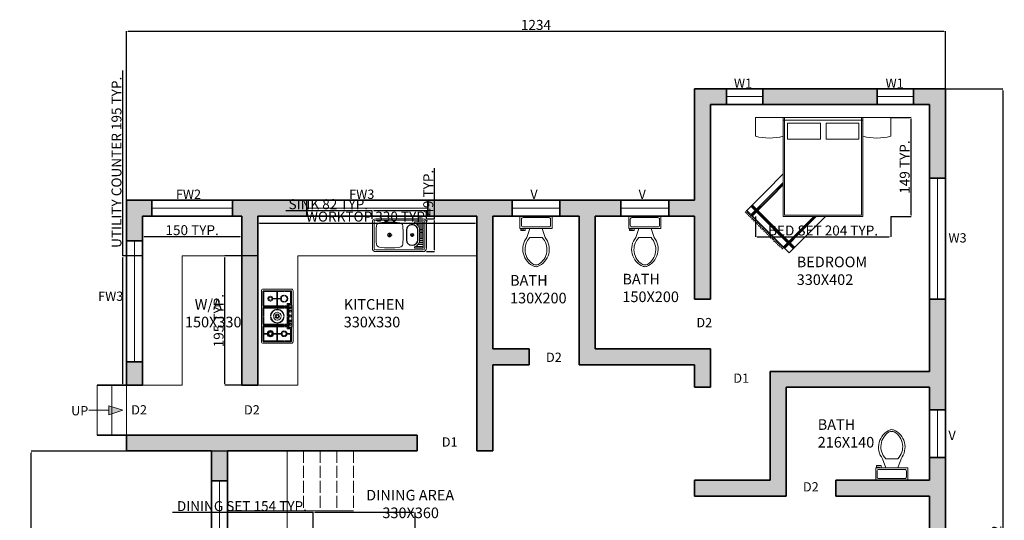
# Model space of a CAD drawing. Units: centimetres. Extents: x 2449 to 7478, y 778 to 2486.
# Tile 6 of 9: x 4189 to 5672, y 1732 to 2486. Entities that reach past the tile are written whole.
import ezdxf

# ---------------------------------------------------------------- set-up
doc = ezdxf.new("R2010")
doc.units = ezdxf.units.CM
doc.linetypes.add('ACAD_ISO02W100', pattern=[15, 12, -3])
for name, color, linetype, lineweight in [('A-ANNO-DIMS', 2, 'Continuous', 18), ('A-ANNO-SYMB', 8, 'Continuous', 18), ('A-ANNO-TEXT', 7, 'Continuous', 18), ('A-AREA-IDEN', 7, 'Continuous', 18), ('A-EQPM', 8, 'Continuous', 18), ('A-FLOR-CASE', 8, 'Continuous', 18), ('A-FLOR-FIXT', 8, 'Continuous', 18), ('A-FLOR-STRS', 7, 'Continuous', 18), ('A-FLOR-STRS-OVHD', 7, 'ACAD_ISO02W100', 13), ('A-WALL', 7, 'Continuous', 35), ('A-WALL-PATT', 7, 'Continuous', 13), ('B-FURNITURE', 22, 'Continuous', 18), ('Win', 1, 'Continuous', 18)]:
    doc.layers.add(name, color=color, linetype=linetype, lineweight=lineweight)
doc.styles.get("Standard").update_dxf_attribs({"font": 'arial.ttf'})
doc.dimstyles.new('ISO-25', dxfattribs={"dimtxt": 15, "dimasz": 2.5, "dimexe": 0, "dimexo": 0, "dimgap": 0, "dimtad": 1, "dimtxsty": 'Standard', "dimcen": 2.5, "dimadec": 0, "dimazin": 0, "dimtfac": 1, "dimtmove": 0, "dimatfit": 3, "dimfxl": 1, "dimarcsym": 0})

# ---------------------------------------------------------------- blocks, each defined once
blk = doc.blocks.new('sink 1')
for points in [[(-7.34, 1.48), (-7.34, 22.73)], [(-6.56, 1.48), (-6.56, 22.73)], [(5.86, 24.22), (-5.86, 24.22)], [(6.01, 23.43), (-5.86, 23.43)], [(6.72, 1.48), (6.72, 22.73)], [(7.34, 1.48), (7.34, 22.73)], [(1.09, 16.48), (-0.94, 16.48)], [(0, 15.39), (0, 17.42)], [(-2.09, 8.99), (2.28, 8.99)], [(-2.09, 8.84), (2.28, 8.84)], [(-5.78, 5.39), (-5.78, 5.39)], [(-5.31, 5.39), (-5.31, 5.39)], [(-5.16, 4.92), (-5.16, 4.92)], [(-5, 1.48), (-5, 4.69)], [(-4.84, 4.45), (-4.84, 4.45)], [(0.78, 6.33), (-0.78, 6.33)], [(0, 5.55), (0, 7.26)], [(5, 4.45), (5, 4.45)], [(5.16, 4.92), (5.16, 4.92)], [(5.94, 5.39), (5.94, 5.39)], [(6.01, 0.78), (-5.86, 0.78)], [(5.86, 0), (-5.86, 0)], [(-5.78, 1.48), (-5.78, 1.48)], [(-5.16, 1.48), (-5.16, 1.48)], [(-5, 1.48), (-4.22, 1.48), (-4.22, 3.83)], [(-4.84, 1.48), (-4.84, 1.48)], [(-4.22, 3.83), (-4.22, 3.83)], [(-4.22, 1.48), (-4.22, 1.48)], [(-4.06, 1.48), (-4.06, 3.69)], [(-4.06, 1.48), (-3.28, 1.48), (-3.28, 3.27)], [(-3.91, 3.52), (-3.91, 3.52)], [(-3.91, 1.48), (-3.91, 1.48)], [(-3.28, 3.2), (-3.28, 3.2)], [(-3.28, 1.48), (-3.28, 1.48)], [(-3.12, 3.2), (-3.12, 3.2)], [(-3.12, 1.48), (-3.12, 1.48)], [(-2.34, 3.05), (-2.34, 3.05)], [(-2.34, 1.48), (-2.34, 1.48)], [(-2.19, 3.05), (-2.19, 3.05)], [(-2.19, 1.48), (-2.19, 1.48)], [(-2.09, 3.99), (2.28, 3.99)], [(-2.09, 3.84), (2.28, 3.84)], [(-1.41, 3.05), (-1.41, 3.05)], [(-1.41, 1.48), (-1.41, 1.48)], [(-1.25, 3.05), (-1.25, 3.05)], [(-0.47, 1.48), (-1.25, 1.48), (-1.25, 3.05), (-0.47, 3.05)], [(-1.25, 1.48), (-1.25, 1.48)], [(-0.62, 3.05), (-0.62, 3.05)], [(-0.62, 1.48), (-0.62, 1.48)], [(-0.47, 1.48), (-0.47, 3.05)], [(-0.31, 3.05), (-0.31, 3.05)], [(0.47, 1.48), (-0.31, 1.48), (-0.31, 3.05), (0.47, 3.05)], [(-0.31, 1.48), (-0.31, 1.48)], [(0.31, 3.05), (0.31, 3.05)], [(0.31, 1.48), (0.31, 1.48)], [(0.47, 1.48), (0.47, 3.05)], [(0.62, 3.05), (0.62, 3.05)], [(0.62, 1.48), (0.62, 1.48)], [(1.25, 3.05), (1.25, 3.05)], [(1.25, 1.48), (1.25, 1.48)], [(1.56, 3.05), (1.56, 3.05)], [(1.56, 1.48), (1.56, 1.48)], [(2.19, 3.05), (2.19, 3.05)], [(2.19, 1.48), (2.19, 1.48)], [(2.5, 3.05), (2.5, 3.05)], [(2.5, 1.48), (2.5, 1.48)], [(3.12, 3.2), (3.12, 3.2)], [(3.12, 1.48), (3.12, 1.48)], [(3.28, 1.48), (4.06, 1.48), (4.06, 3.57)], [(3.28, 1.48), (3.28, 3.2)], [(3.44, 3.2), (3.44, 3.2)], [(3.44, 1.48), (3.44, 1.48)], [(4.06, 3.52), (4.06, 3.52)], [(4.06, 1.48), (4.06, 1.48)], [(4.22, 1.48), (4.22, 3.67)], [(4.37, 3.83), (4.37, 3.83)], [(4.37, 1.48), (4.37, 1.48)], [(5, 1.48), (5, 1.48)], [(5.16, 1.48), (5.16, 1.48)], [(5.94, 1.48), (5.94, 1.48)]]:
    blk.add_lwpolyline(points)
for points in [[(-5.16, 4.92), (-5.16, 1.48), (-5.78, 1.48), (-5.78, 5.39), (-5.31, 5.39, -0.068511), (-5.16, 4.92)], [(4.22, 1.48), (5, 1.48), (5, 4.45, -0.083542), (4.22, 3.67, -0.083542)], [(5.16, 4.92, 0.248301), (5.47, 5.39), (5.94, 5.39), (5.94, 1.48), (5.16, 1.48), (5.16, 4.92)], [(4.06, 3.57, -0.061679), (3.32, 3.22)]]:
    blk.add_lwpolyline(points, format="xyb")
for points in [[(-3.12, 3.22), (-3.12, 1.48), (-2.34, 1.48), (-2.34, 3.05, -0.06228)], [(2.5, 3.05), (2.5, 1.48), (3.12, 1.48), (3.12, 3.2, -0.050256)]]:
    blk.add_lwpolyline(points, format="xyb", close=True)
for points in [[(-2.19, 3.05), (-1.41, 3.05), (-1.41, 1.48), (-2.19, 1.48)], [(0.62, 3.05), (1.25, 3.05), (1.25, 1.48), (0.62, 1.48)], [(2.19, 1.48), (2.19, 3.05), (1.56, 3.05), (1.56, 1.48)]]:
    blk.add_lwpolyline(points, close=True)
for centre, radius in [((0.09, 16.57), 0.859), ((0.09, 16.57), 0.703), ((0.09, 6.41), 0.703), ((0.09, 6.41), 0.547)]:
    blk.add_circle(centre, radius)
for centre, radius, start, end in [((-5.86, 22.73), 1.48, 90, 180), ((-5.86, 22.73), 0.703, 90, 180), ((-3.87, 20.82), 1.53, 97.3256, 171.1849), ((0.09, -12.65), 35.23, 83.2159, 96.7841), ((4.06, 20.82), 1.53, 8.8151, 82.6744), ((5.86, 22.73), 1.48, 360, 90), ((6.01, 22.73), 0.703, 0, 90), ((30.19, 16.56), 35.85, 172.7947, 187.4213), ((-30, 16.56), 35.85, 352.5787, 7.2053), ((-3.89, 12.12), 1.48, 187.4212, 263.2159), ((-2.1, 6.41), 2.58, 90, 270), ((-2.1, 6.41), 2.42, 90, 270), ((0.09, 45.63), 35.23, 263.2159, 276.7841), ((2.28, 6.41), 2.58, 270, 90), ((2.28, 6.41), 2.42, 270, 90), ((4.08, 12.12), 1.48, 276.7841, 352.5788), ((-2.15, 6.48), 3.36, 212.1095, 232.0862), ((-5.86, 1.48), 1.48, 180, 270), ((-5.86, 1.48), 0.703, 180, 270), ((-2.1, 6.41), 3.36, 234.156, 249.3275), ((2.14, 6.36), 3.36, 289.8633, 290.5971), ((5.86, 1.48), 1.48, 270, 0), ((6.01, 1.48), 0.703, 270, 360)]:
    blk.add_arc(centre, radius, start, end)
blk = doc.blocks.new('STOVE')
for p, q in [((11.85, 19.7), (11.55, 19.7)), ((11.55, 16.92), (11.55, 19.7)), ((11.85, 16.92), (11.85, 19.7)), ((-11.85, 13.73), (-11.85, 7.62)), ((-11.85, 13.73), (-11.55, 13.73)), ((-11.55, 13.73), (-11.55, 7.62)), ((11.85, 16.92), (11.55, 16.92)), ((11.85, 13.23), (11.55, 13.23)), ((11.55, 13.23), (11.55, 7.57)), ((11.85, 13.23), (11.85, 7.57)), ((-11.85, 10.75), (-16.4, 10.75)), ((-11.85, 10.25), (-16.4, 10.25)), ((-11.85, 7.62), (-11.55, 7.62)), ((-7, 10.75), (-11.55, 10.75)), ((-7, 10.25), (-11.55, 10.25)), ((7, 10.75), (11.55, 10.75)), ((7, 10.25), (11.55, 10.25)), ((11.85, 7.57), (11.55, 7.57)), ((11.85, 10.75), (16.4, 10.75)), ((11.85, 10.25), (16.4, 10.25)), ((-7, 3.9), (-8.4, 3.9)), ((-7.8, 3.3), (-7.8, 1)), ((-6.4, 3.3), (-7.8, 3.3)), ((7.3, 2.8), (-7.3, 2.8)), ((-7.3, 2.8), (-7.3, 0.8)), ((7.3, 0.8), (-7.3, 0.8)), ((-5.4, 3.9), (-6, 3.9)), ((-5.4, 3.9), (-0.15, 3.9)), ((0.15, 3.9), (5.4, 3.9)), ((6.4, 3.3), (7.8, 3.3)), ((7, 3.9), (8.4, 3.9)), ((7.3, 2.8), (7.3, 0.8)), ((7.8, 3.3), (7.8, 1)), ((8.4, 3.9), (8.4, 1.6)), ((11.85, 4.28), (11.55, 4.28)), ((11.55, 4.28), (11.55, 1.3)), ((11.85, 1.3), (11.55, 1.3)), ((11.85, 4.28), (11.85, 1.3))]:
    blk.add_line(p, q)
for points in [[(-17, 21), (17, 21, -0.414214), (18, 20), (18, 1, -0.414214), (17, 0), (-17, 0, -0.414214), (-18, 1), (-18, 20, -0.414214)], [(6, 3.3), (-6, 3.3), (-6, 19.4, -0.414214), (-5.4, 20), (5.4, 20, -0.414214), (6, 19.4)]]:
    blk.add_lwpolyline(points, format="xyb", close=True)
for points in [[(-7.8, 1), (-16.4, 1, -0.414214), (-17, 1.6), (-17, 19.4, -0.414214), (-16.4, 20), (-7, 20, -0.414214), (-6.4, 19.4), (-6.4, 3.3)], [(6.4, 19.4, -0.414214), (7, 20), (16.4, 20, -0.414214), (17, 19.4), (17, 1.6, -0.414214), (16.4, 1), (7.8, 1)]]:
    blk.add_lwpolyline(points, format="xyb")
for points in [[(-16.4, 15.22), (-16.4, 19.4), (-11.85, 19.4)], [(-16.4, 6.08), (-16.4, 14.92)], [(-11.55, 19.4), (-7, 19.4), (-7, 15.22)], [(-7, 14.92), (-7, 6.08)], [(-5.4, 15.22), (-5.4, 19.4), (-0.15, 19.4)], [(-5.4, 10.65), (-5.4, 14.92)], [(0.15, 19.4), (5.4, 19.4), (5.4, 15.22)], [(5.4, 14.92), (5.4, 10.65)], [(6.4, 3.3), (6.4, 19.4)], [(7, 15.22), (7, 19.4), (11.55, 19.4)], [(7, 6.08), (7, 14.92)], [(11.85, 19.4), (16.4, 19.4), (16.4, 15.22)], [(16.4, 14.92), (16.4, 6.08)], [(-5.4, 6.08), (-5.4, 10.35)], [(5.4, 10.35), (5.4, 6.08)], [(-11.85, 1.6), (-16.4, 1.6), (-16.4, 5.77)], [(-8.4, 3.9), (-8.4, 1.6), (-11.55, 1.6)], [(-7, 5.77), (-7, 3.9)], [(-5.4, 3.9), (-5.4, 5.77)], [(5.4, 5.77), (5.4, 3.9)], [(7, 3.9), (7, 5.77)], [(11.55, 1.6), (8.4, 1.6)], [(16.4, 5.77), (16.4, 1.6), (11.85, 1.6)]]:
    blk.add_lwpolyline(points)
for centre, radius in [((-11.7, 15.07), 1.1), ((11.7, 15.07), 1.6), ((11.7, 15.07), 1.1), ((0, 10.5), 1.4), ((0, 10.5), 0.8), ((11.7, 5.93), 1.4), ((-5.49, 1.8), 0.6), ((-3.3, 1.8), 0.6), ((0, 1.8), 0.6), ((3.39, 1.8), 0.6), ((5.57, 1.8), 0.6)]:
    blk.add_circle(centre, radius)
for centre, radius, start, end in [((-11.7, 15.07), 1.6, 95.37938, 174.62062), ((-11.7, 15.07), 1.6, 185.37938, 264.62062), ((-11.7, 15.07), 1.6, 5.37938, 84.62062), ((-11.7, 15.07), 1.6, 275.37938, 354.62062), ((0, 10.5), 4.6, 91.86867, 178.13133), ((0, 10.5), 4.3, 91.9991, 178.0009), ((0, 10.5), 4.6, 1.86867, 88.13133), ((0, 10.5), 4.3, 1.9991, 88.0009), ((11.7, 15.07), 2.1, 94.09604, 175.90396), ((11.7, 15.07), 2.1, 184.09604, 265.90396), ((11.7, 15.07), 2.1, 4.09604, 85.90396), ((11.7, 15.07), 2.1, 274.09604, 355.90396), ((-11.7, 5.93), 2.4, 93.58332, 176.41668), ((-11.7, 5.93), 2, 94.30122, 175.69878), ((-11.7, 5.93), 2.4, 3.58332, 86.41668), ((-11.7, 5.93), 2, 4.30122, 85.69878), ((0, 10.5), 4.6, 181.86867, 268.13133), ((0, 10.5), 4.3, 181.9991, 268.0009), ((0, 10.5), 2.6, 93.30736, 176.69264), ((0, 10.5), 2.6, 183.30736, 266.69264), ((0, 10.5), 2.6, 3.30736, 86.69264), ((0, 10.5), 4.6, 271.86867, 358.13133), ((0, 10.5), 4.3, 271.9991, 358.0009), ((0, 10.5), 2.6, 273.30736, 356.69264), ((11.7, 5.93), 1.9, 94.52806, 175.47194), ((11.7, 5.93), 1.9, 4.52806, 85.47194), ((-11.7, 5.93), 2.4, 183.58332, 266.41668), ((-11.7, 5.93), 2, 184.30122, 265.69878), ((-11.7, 5.93), 2.4, 273.58332, 356.41668), ((-11.7, 5.93), 2, 274.30122, 355.69878), ((-5.49, 1.8), 0.846, 89.99794, 270), ((-3.3, 1.8), 0.846, 89.99794, 270), ((0, 1.8), 0.846, 89.99794, 270), ((3.39, 1.8), 0.846, 89.99794, 270), ((5.57, 1.8), 0.846, 89.99794, 270), ((11.7, 5.93), 1.9, 184.52806, 265.47194), ((11.7, 5.93), 1.9, 274.52806, 355.47194)]:
    blk.add_arc(centre, radius, start, end)
blk = doc.blocks.new('Toilet - top')
for p, q in [((9.5, -6), (9.5, -2)), ((-10, -8.5), (-8, -8.5)), ((-10, -9.5), (-10, -8.5)), ((-7, -9.5), (-10, -9.5)), ((-8, -8.5), (-8, -8)), ((-7, -8), (-7, -9.5)), ((-4, -8), (-6, -14)), ((4, -8), (6, -14)), ((4, -14), (-4, -14))]:
    blk.add_line(p, q)
blk.add_lwpolyline([(10.5, -8), (10.5, 0), (-10.5, 0), (-10.5, -8)], close=True)
for points in [[(-9.5, -2), (-9.5, -6)], [(8.5, -1), (-8.5, -1)], [(-8.5, -7), (8.5, -7)]]:
    blk.add_lwpolyline(points)
for centre, radius, start, end in [((-8.62, -1.88), 0.884, 81.8699, 188.1301), ((-8.62, -6.12), 0.884, 171.8699, 278.1301), ((8.62, -1.88), 0.884, 351.8699, 98.1301), ((8.62, -6.12), 0.884, 261.8699, 8.1301), ((3.52, -21.58), 12.17, 141.46911, 247.97143), ((4.2, -21.82), 11.33, 136.36773, 238.94682), ((-3.52, -21.58), 12.17, 292.02843, 38.53071), ((-4.2, -21.82), 11.33, 301.05301, 43.63209), ((0, -27.88), 4, 245.73182, 294.26817), ((0, -29), 4, 254.86053, 285.13947)]:
    blk.add_arc(centre, radius, start, end)
blk = doc.blocks.new('A$C376C2187')
at = {"layer": 'B-FURNITURE'}
for p, q in [((-1.53, 1.82), (-1.53, 2.24)), ((-1.53, 2.24), (-0.9, 2.24)), ((-0.9, 0), (-0.9, 2.24)), ((-0.9, 2.24), (0.9, 2.24)), ((-0.9, 2.24), (-0.9, 1.82)), ((-0.87, 0.03), (-0.87, 2.24)), ((0.87, 2.24), (0.87, 0.03)), ((0.9, 2.24), (0.9, 0)), ((0.9, 1.82), (0.9, 2.24)), ((0.9, 2.24), (1.53, 2.24)), ((1.53, 2.24), (1.53, 1.82)), ((-0.9, 2.182), (0.9, 2.182)), ((-0.807, 2.112), (-0.057, 2.112)), ((-0.807, 1.749), (-0.807, 2.112)), ((-0.057, 2.112), (-0.057, 1.749)), ((0.069, 2.112), (0.807, 2.112)), ((0.069, 2.112), (0.069, 1.749)), ((0.807, 2.112), (0.807, 1.749)), ((-0.807, 1.749), (-0.057, 1.749)), ((0.069, 1.749), (0.807, 1.749)), ((0.9, 0), (-0.9, 0)), ((0.87, 0.03), (-0.87, 0.03))]:
    blk.add_line(p, q, dxfattribs=at)
for centre in [(-1.215, 2.926), (1.215, 2.926)]:
    blk.add_arc(centre, 1.15, 254.0965, 285.9035, dxfattribs=at)
blk = doc.blocks.new('RUG-FRINGED-A')
for p, q in [((57.6, 119.1), (31.1, 92.6)), ((37.5, 86.2), (57.6, 106.3)), ((2.5, 63.9), (31.1, 92.6)), ((38.9, 84.8), (57.6, 103.6)), ((39.5, 84.2), (57.6, 102.4)), ((37.5, 86.2), (8.9, 57.6)), ((38.9, 84.8), (10.3, 56.2)), ((39.5, 84.2), (10.8, 55.6)), ((2.6, 63.8), (0, 61.2)), ((4.3, 62.2), (1.7, 59.5)), ((66.5, 0), (2.5, 63.9)), ((6, 60.5), (3.4, 57.9)), ((72.9, 6.4), (8.9, 70.3)), ((74.2, 7.7), (10.3, 71.7)), ((74.8, 8.3), (10.8, 72.3)), ((7.7, 58.8), (5, 56.2)), ((9.3, 57.1), (6.7, 54.5)), ((11, 55.4), (8.4, 52.8)), ((12.7, 53.8), (10.1, 51.1)), ((14.4, 52.1), (11.8, 49.5)), ((16.1, 50.4), (13.4, 47.8)), ((17.7, 48.7), (15.1, 46.1)), ((19.4, 47), (16.8, 44.4)), ((21.1, 45.4), (18.5, 42.7)), ((103.4, 54.7), (86.2, 37.5)), ((104.6, 54.7), (86.8, 36.9)), ((107.3, 54.7), (88.1, 35.6)), ((95.1, 28.6), (121.2, 54.7)), ((22.8, 43.7), (20.2, 41.1)), ((24.5, 42), (21.8, 39.4)), ((26.1, 40.3), (23.5, 37.7)), ((27.8, 38.6), (25.2, 36)), ((29.5, 37), (26.9, 34.3)), ((31.2, 35.3), (28.6, 32.7)), ((32.9, 33.6), (30.2, 31)), ((34.5, 31.9), (31.9, 29.3)), ((36.2, 30.2), (33.6, 27.6)), ((57.6, 8.9), (86.2, 37.5)), ((58.2, 8.3), (86.8, 36.9)), ((59.5, 6.9), (88.1, 35.6)), ((37.9, 28.6), (35.3, 25.9)), ((39.6, 26.9), (37, 24.3)), ((41.3, 25.2), (38.6, 22.6)), ((42.9, 23.5), (40.3, 20.9)), ((44.6, 21.8), (42, 19.2)), ((46.3, 20.2), (43.7, 17.5)), ((48, 18.5), (45.4, 15.9)), ((49.7, 16.8), (47, 14.2)), ((51.3, 15.1), (48.7, 12.5)), ((95.1, 28.6), (66.5, 0)), ((53, 13.4), (50.4, 10.8)), ((54.7, 11.8), (52.1, 9.1)), ((56.4, 10.1), (53.8, 7.5)), ((58.1, 8.4), (55.4, 5.8))]:
    blk.add_line(p, q)
for centre in [(1.6, 59.5), (3.3, 57.8), (5, 56.1), (6.7, 54.4), (8.3, 52.8), (10, 51.1), (11.7, 49.4), (13.4, 47.7), (15.1, 46), (16.7, 44.4), (18.4, 42.7), (20.1, 41), (21.8, 39.3), (23.5, 37.6), (25.1, 36), (26.8, 34.3), (28.5, 32.6), (30.2, 30.9), (31.9, 29.2), (33.5, 27.6), (35.2, 25.9), (36.9, 24.2), (38.6, 22.5), (40.3, 20.8), (41.9, 19.2), (43.6, 17.5), (45.3, 15.8), (47, 14.1), (48.7, 12.4), (50.3, 10.8), (52, 9.1)]:
    blk.add_circle(centre, 0.0789)
blk = doc.blocks.new('COUNTER-KITCHEN')
for p, q in [((0, 0), (270, 0)), ((0, 0), (0, -195)), ((0, -195), (-60, -195))]:
    blk.add_line(p, q)
blk = doc.blocks.new('COUNTER-UTILITY')
for p, q in [((0, 0), (90, 0)), ((0, 0), (0, -195)), ((-60, -195), (0, -195))]:
    blk.add_line(p, q)
blk = doc.blocks.new('ARROW-ENTRY-UP')
at = {"transparency": 33554687}
h = blk.add_hatch(color=256, dxfattribs=at)
h.dxf.hatch_style = 1
h.paths.add_polyline_path([(-6.8, 30.3), (6.8, 30.3), (0, 51.2)])
blk.add_line((0, 30.3), (0, 0))
blk.add_lwpolyline([(0, 51.2), (-6.8, 30.3), (6.8, 30.3)], close=True)
blk = doc.blocks.new('*D80')
at = {"layer": 'A-ANNO-DIMS', "color": 0, "lineweight": -2, "transparency": 16777216}
for p, q in [((5297.1, 2189.5), (5297.1, 2158.9)), ((5501, 2189.5), (5501, 2158.9)), ((5299.6, 2158.9), (5498.5, 2158.9))]:
    blk.add_line(p, q, dxfattribs=at)
at = {"layer": 'A-ANNO-DIMS', "color": 0, "transparency": 16777216}
for points in [[(5299.6, 2159.4), (5299.6, 2158.5), (5297.1, 2158.9)], [(5498.5, 2159.4), (5498.5, 2158.5), (5501, 2158.9)]]:
    blk.add_solid(points, dxfattribs=at)
at = {"layer": 'Defpoints', "color": 0, "transparency": 16777216}
for p in [(5297.1, 2189.5), (5501, 2189.5), (5501, 2158.9)]:
    blk.add_point(p, dxfattribs=at)
at = {"layer": 'A-ANNO-DIMS', "color": 0, "transparency": 16777216, "insert": (5399.1, 2166.7), "char_height": 15, "attachment_point": 5}
blk.add_mtext('BED SET 204 TYP.', dxfattribs=at)
blk = doc.blocks.new('*D81')
at = {"layer": 'A-ANNO-DIMS', "color": 0, "lineweight": -2, "transparency": 16777216}
for p, q in [((5501, 2338.8), (5531.6, 2338.8)), ((5531.6, 2192), (5531.6, 2336.3)), ((5501, 2189.5), (5531.6, 2189.5))]:
    blk.add_line(p, q, dxfattribs=at)
at = {"layer": 'A-ANNO-DIMS', "color": 0, "transparency": 16777216}
for points in [[(5531.2, 2336.3), (5532.1, 2336.3), (5531.6, 2338.8)], [(5531.2, 2192), (5532.1, 2192), (5531.6, 2189.5)]]:
    blk.add_solid(points, dxfattribs=at)
at = {"layer": 'Defpoints', "color": 0, "transparency": 16777216}
for p in [(5501, 2338.8), (5531.6, 2338.8), (5501, 2189.5)]:
    blk.add_point(p, dxfattribs=at)
at = {"layer": 'A-ANNO-DIMS', "color": 0, "transparency": 16777216, "insert": (5524, 2264.2), "char_height": 15, "attachment_point": 5, "rotation": 90}
blk.add_mtext('149 TYP.', dxfattribs=at)
blk = doc.blocks.new('*D88')
at = {"layer": 'A-ANNO-DIMS', "color": 0, "lineweight": -2, "transparency": 16777216}
for p, q in [((4630.8, 1743.6), (4418.6, 1743.6)), ((4630.8, 1720.5), (4630.8, 1743.6)), ((4781.9, 1743.6), (4633.3, 1743.6)), ((4784.4, 1720.5), (4784.4, 1743.6))]:
    blk.add_line(p, q, dxfattribs=at)
at = {"layer": 'A-ANNO-DIMS', "color": 0, "transparency": 16777216}
for points in [[(4633.3, 1744), (4633.3, 1743.2), (4630.8, 1743.6)], [(4781.9, 1744), (4781.9, 1743.2), (4784.4, 1743.6)]]:
    blk.add_solid(points, dxfattribs=at)
at = {"layer": 'Defpoints', "color": 0, "transparency": 16777216}
for p in [(4630.8, 1743.6), (4630.8, 1720.5), (4784.4, 1720.5)]:
    blk.add_point(p, dxfattribs=at)
at = {"layer": 'A-ANNO-DIMS', "color": 0, "transparency": 16777216, "insert": (4523.4, 1751.3), "char_height": 15, "attachment_point": 5}
blk.add_mtext('DINING SET 154 TYP.', dxfattribs=at)
blk = doc.blocks.new('*D90')
at = {"layer": 'A-ANNO-DIMS', "color": 0, "lineweight": -2, "transparency": 16777216}
for p, q in [((4719.9, 2198.5), (4589.8, 2198.5)), ((4719.9, 2186.3), (4719.9, 2198.5)), ((4799, 2198.5), (4722.4, 2198.5)), ((4801.5, 2186.3), (4801.5, 2198.5))]:
    blk.add_line(p, q, dxfattribs=at)
at = {"layer": 'A-ANNO-DIMS', "color": 0, "transparency": 16777216}
for points in [[(4722.4, 2199), (4722.4, 2198.1), (4719.9, 2198.5)], [(4799, 2199), (4799, 2198.1), (4801.5, 2198.5)]]:
    blk.add_solid(points, dxfattribs=at)
at = {"layer": 'Defpoints', "color": 0, "transparency": 16777216}
for p in [(4719.9, 2198.5), (4719.9, 2186.3), (4801.5, 2186.3)]:
    blk.add_point(p, dxfattribs=at)
at = {"layer": 'A-ANNO-DIMS', "color": 0, "transparency": 16777216, "insert": (4653.6, 2206.3), "char_height": 15, "attachment_point": 5}
blk.add_mtext('SINK 82 TYP.', dxfattribs=at)
blk = doc.blocks.new('*D91')
at = {"layer": 'A-ANNO-DIMS', "color": 0, "lineweight": -2, "transparency": 16777216}
for p, q in [((4813.7, 2186.3), (4813.7, 2262.4)), ((4801.5, 2186.3), (4813.7, 2186.3)), ((4813.7, 2139.3), (4813.7, 2183.8)), ((4801.5, 2136.8), (4813.7, 2136.8))]:
    blk.add_line(p, q, dxfattribs=at)
at = {"layer": 'A-ANNO-DIMS', "color": 0, "transparency": 16777216}
for points in [[(4813.3, 2183.8), (4814.1, 2183.8), (4813.7, 2186.3)], [(4813.3, 2139.3), (4814.1, 2139.3), (4813.7, 2136.8)]]:
    blk.add_solid(points, dxfattribs=at)
at = {"layer": 'Defpoints', "color": 0, "transparency": 16777216}
for p in [(4801.5, 2186.3), (4813.7, 2186.3), (4801.5, 2136.8)]:
    blk.add_point(p, dxfattribs=at)
at = {"layer": 'A-ANNO-DIMS', "color": 0, "transparency": 16777216, "insert": (4806.1, 2225.6), "char_height": 15, "attachment_point": 5, "rotation": 90}
blk.add_mtext('49 TYP.', dxfattribs=at)
blk = doc.blocks.new('*D96')
at = {"layer": 'A-ANNO-DIMS', "color": 0, "lineweight": -2, "transparency": 16777216}
for p, q in [((4547.4, 2130.3), (4547.4, 2179.8)), ((4549.9, 2179.8), (4874.9, 2179.8)), ((4877.4, 2130.3), (4877.4, 2179.8))]:
    blk.add_line(p, q, dxfattribs=at)
at = {"layer": 'A-ANNO-DIMS', "color": 0, "transparency": 16777216}
for points in [[(4549.9, 2180.3), (4549.9, 2179.4), (4547.4, 2179.8)], [(4874.9, 2180.3), (4874.9, 2179.4), (4877.4, 2179.8)]]:
    blk.add_solid(points, dxfattribs=at)
at = {"layer": 'Defpoints', "color": 0, "transparency": 16777216}
for p in [(4877.4, 2179.8), (4547.4, 2130.3), (4877.4, 2130.3)]:
    blk.add_point(p, dxfattribs=at)
at = {"layer": 'A-ANNO-DIMS', "color": 0, "transparency": 16777216, "insert": (4712.4, 2187.6), "char_height": 15, "attachment_point": 5}
blk.add_mtext('WORKTOP 330 TYP.', dxfattribs=at)
blk = doc.blocks.new('*D97')
at = {"layer": 'A-ANNO-DIMS', "color": 0, "lineweight": -2, "transparency": 16777216}
for p, q in [((4547.4, 2130.3), (4497.9, 2130.3)), ((4497.9, 1937.8), (4497.9, 2127.8)), ((4547.4, 1935.3), (4497.9, 1935.3))]:
    blk.add_line(p, q, dxfattribs=at)
at = {"layer": 'A-ANNO-DIMS', "color": 0, "transparency": 16777216}
for points in [[(4497.5, 2127.8), (4498.4, 2127.8), (4497.9, 2130.3)], [(4497.5, 1937.8), (4498.4, 1937.8), (4497.9, 1935.3)]]:
    blk.add_solid(points, dxfattribs=at)
at = {"layer": 'Defpoints', "color": 0, "transparency": 16777216}
for p in [(4497.9, 2130.3), (4547.4, 2130.3), (4547.4, 1935.3)]:
    blk.add_point(p, dxfattribs=at)
at = {"layer": 'A-ANNO-DIMS', "color": 0, "transparency": 16777216, "insert": (4490.3, 2032.8), "char_height": 15, "attachment_point": 5, "rotation": 90}
blk.add_mtext('195 TYP.', dxfattribs=at)
blk = doc.blocks.new('*D98')
at = {"layer": 'A-ANNO-DIMS', "color": 0, "lineweight": -2, "transparency": 16777216}
for p, q in [((4344.2, 2130.3), (4344.2, 2410)), ((4373.4, 2130.3), (4344.2, 2130.3)), ((4344.2, 1937.8), (4344.2, 2127.8)), ((4373.4, 1935.3), (4344.2, 1935.3))]:
    blk.add_line(p, q, dxfattribs=at)
at = {"layer": 'A-ANNO-DIMS', "color": 0, "transparency": 16777216}
for points in [[(4343.8, 2127.8), (4344.6, 2127.8), (4344.2, 2130.3)], [(4343.8, 1937.8), (4344.6, 1937.8), (4344.2, 1935.3)]]:
    blk.add_solid(points, dxfattribs=at)
at = {"layer": 'Defpoints', "color": 0, "transparency": 16777216}
for p in [(4344.2, 2130.3), (4373.4, 2130.3), (4373.4, 1935.3)]:
    blk.add_point(p, dxfattribs=at)
at = {"layer": 'A-ANNO-DIMS', "color": 0, "transparency": 16777216, "insert": (4336.4, 2271.4), "char_height": 15, "attachment_point": 5, "rotation": 90}
blk.add_mtext('UTILITY COUNTER 195 TYP.', dxfattribs=at)
blk = doc.blocks.new('*D99')
at = {"layer": 'A-ANNO-DIMS', "color": 0, "lineweight": -2, "transparency": 16777216}
for p, q in [((4373.4, 2130.3), (4373.4, 2159.6)), ((4375.9, 2159.6), (4520.9, 2159.6)), ((4523.4, 2130.3), (4523.4, 2159.6))]:
    blk.add_line(p, q, dxfattribs=at)
at = {"layer": 'A-ANNO-DIMS', "color": 0, "transparency": 16777216}
for points in [[(4375.9, 2160), (4375.9, 2159.2), (4373.4, 2159.6)], [(4520.9, 2160), (4520.9, 2159.2), (4523.4, 2159.6)]]:
    blk.add_solid(points, dxfattribs=at)
at = {"layer": 'Defpoints', "color": 0, "transparency": 16777216}
for p in [(4523.4, 2159.6), (4373.4, 2130.3), (4523.4, 2130.3)]:
    blk.add_point(p, dxfattribs=at)
at = {"layer": 'A-ANNO-DIMS', "color": 0, "transparency": 16777216, "insert": (4448.4, 2167.2), "char_height": 15, "attachment_point": 5}
blk.add_mtext('150 TYP.', dxfattribs=at)
blk = doc.blocks.new('*D100')
at = {"layer": 'A-ANNO-DIMS', "color": 0, "lineweight": -2, "transparency": 16777216}
for p, q in [((4349.4, 2214.3), (4349.4, 2468.8)), ((4351.9, 2468.8), (5580.9, 2468.8)), ((5583.4, 2382.3), (5583.4, 2468.8))]:
    blk.add_line(p, q, dxfattribs=at)
at = {"layer": 'A-ANNO-DIMS', "color": 0, "transparency": 16777216}
for points in [[(4351.9, 2469.3), (4351.9, 2468.4), (4349.4, 2468.8)], [(5580.9, 2469.3), (5580.9, 2468.4), (5583.4, 2468.8)]]:
    blk.add_solid(points, dxfattribs=at)
at = {"layer": 'Defpoints', "color": 0, "transparency": 16777216}
for p in [(5583.4, 2468.8), (5583.4, 2382.3), (4349.4, 2214.3)]:
    blk.add_point(p, dxfattribs=at)
at = {"layer": 'A-ANNO-DIMS', "color": 0, "transparency": 16777216, "insert": (4966.4, 2476.5), "char_height": 15, "attachment_point": 5}
blk.add_mtext('1234', dxfattribs=at)
blk = doc.blocks.new('*D101')
at = {"layer": 'A-ANNO-DIMS', "color": 0, "lineweight": -2, "transparency": 16777216}
for p, q in [((5583.4, 2382.3), (5669.9, 2382.3)), ((5669.9, 2379.8), (5669.9, 1022.8)), ((5583.4, 1020.3), (5669.9, 1020.3))]:
    blk.add_line(p, q, dxfattribs=at)
at = {"layer": 'A-ANNO-DIMS', "color": 0, "transparency": 16777216}
for points in [[(5669.5, 2379.8), (5670.4, 2379.8), (5669.9, 2382.3)], [(5669.5, 1022.8), (5670.4, 1022.8), (5669.9, 1020.3)]]:
    blk.add_solid(points, dxfattribs=at)
at = {"layer": 'Defpoints', "color": 0, "transparency": 16777216}
for p in [(5583.4, 2382.3), (5583.4, 1020.3), (5669.9, 1020.3)]:
    blk.add_point(p, dxfattribs=at)
at = {"layer": 'A-ANNO-DIMS', "color": 0, "transparency": 16777216, "insert": (5662.3, 1701.3), "char_height": 15, "attachment_point": 5, "rotation": 90}
blk.add_mtext('1362', dxfattribs=at)
blk = doc.blocks.new('*D104')
at = {"layer": 'A-ANNO-DIMS', "color": 0, "lineweight": -2, "transparency": 16777216}
for p, q in [((4501.4, 1836.3), (4206.1, 1836.3)), ((4206.1, 1478.8), (4206.1, 1833.8)), ((4501.4, 1476.3), (4206.1, 1476.3))]:
    blk.add_line(p, q, dxfattribs=at)
at = {"layer": 'A-ANNO-DIMS', "color": 0, "transparency": 16777216}
for points in [[(4205.7, 1833.8), (4206.5, 1833.8), (4206.1, 1836.3)], [(4205.7, 1478.8), (4206.5, 1478.8), (4206.1, 1476.3)]]:
    blk.add_solid(points, dxfattribs=at)
at = {"layer": 'Defpoints', "color": 0, "transparency": 16777216}
for p in [(4206.1, 1836.3), (4501.4, 1836.3), (4501.4, 1476.3)]:
    blk.add_point(p, dxfattribs=at)
at = {"layer": 'A-ANNO-DIMS', "color": 0, "transparency": 16777216, "insert": (4198.4, 1656.3), "char_height": 15, "attachment_point": 5, "rotation": 90}
blk.add_mtext('360', dxfattribs=at)

msp = doc.modelspace()

# ---------------------------------------------------------------- hatches: boundary and pattern name
at = {"layer": 'A-WALL-PATT'}
h = msp.add_hatch(color=256, dxfattribs=at)
h.dxf.hatch_style = 1
h.paths.add_polyline_path([(4831.448, 1092.34), (4757.448, 1092.34), (4757.448, 1068.34), (4855.448, 1068.34), (4855.448, 1476.34), (4831.448, 1476.34)])
h.paths.add_polyline_path([(4477.448, 1167.34), (4501.448, 1167.34), (4501.448, 1377.34), (4477.448, 1377.34)])
h.paths.add_polyline_path([(4575.448, 1068.34), (4575.448, 1092.34), (4501.448, 1092.34), (4501.448, 1112.34), (4477.448, 1112.34), (4477.448, 1068.34)])
h.paths.add_polyline_path([(4501.448, 1551.34), (4477.448, 1551.34), (4477.448, 1432.34), (4501.448, 1432.34), (4501.448, 1452.34), (4741.448, 1452.34), (4741.448, 1476.34), (4501.448, 1476.34)])
h.paths.add_polyline_path([(5205.448, 1654.34), (5205.448, 1266.34), (5176.448, 1266.34), (5176.448, 1242.34), (5229.448, 1242.34), (5229.448, 1404.34), (5253.448, 1404.34), (5253.448, 1428.34), (5229.448, 1428.34), (5229.448, 1678.34), (5031.448, 1678.34), (5031.448, 1654.34)])
h.paths.add_polyline_path([(4994.448, 1266.34), (4965.448, 1266.34), (4965.448, 1242.34), (4994.448, 1242.34)])
h.paths.add_polyline_path([(5583.448, 1506.339), (5559.448, 1506.339), (5559.448, 1428.34), (5535.448, 1428.34), (5535.448, 1404.34), (5583.448, 1404.34)])
h.paths.add_polyline_path([(5480.448, 1404.34), (5480.448, 1428.34), (5308.448, 1428.34), (5308.448, 1404.34)])
h.paths.add_polyline_path([(5559.448, 1688.339), (5583.448, 1688.339), (5583.448, 1826.34), (5559.448, 1826.34), (5559.448, 1792.34), (5418.448, 1792.34), (5418.448, 1768.34), (5559.448, 1768.34)])
h.paths.add_polyline_path([(5559.448, 1956.34), (5319.448, 1956.34), (5319.448, 1792.34), (5205.448, 1792.34), (5205.448, 1768.34), (5343.448, 1768.34), (5343.448, 1932.34), (5559.448, 1932.34), (5559.448, 1898.34), (5583.448, 1898.34), (5583.448, 2065.339), (5559.448, 2065.339)])
h.paths.add_polyline_path([(5559.448, 2358.34), (5559.448, 2247.339), (5583.448, 2247.339), (5583.448, 2382.34), (5535.448, 2382.34), (5535.448, 2358.34)])
h.paths.add_polyline_path([(5308.448, 2382.34), (5308.448, 2358.34), (5480.448, 2358.34), (5480.448, 2382.34)])
h.paths.add_polyline_path([(5229.448, 2358.34), (5253.448, 2358.34), (5253.448, 2382.34), (5205.448, 2382.34), (5205.448, 2214.34), (5166.448, 2214.34), (5166.448, 2190.34), (5205.448, 2190.34), (5205.448, 2065.34), (5229.448, 2065.34)])
h.paths.add_polyline_path([(5002.448, 2214.34), (5002.448, 2190.34), (5031.448, 2190.34), (5031.448, 1966.34), (5205.448, 1966.34), (5205.448, 1932.34), (5229.448, 1932.34), (5229.448, 1990.34), (5055.448, 1990.34), (5055.448, 2190.34), (5094.448, 2190.34), (5094.448, 2214.34)])
h.paths.add_polyline_path([(4901.448, 2190.34), (4930.448, 2190.34), (4930.448, 2214.34), (4803.448, 2214.34), (4803.448, 2190.34), (4877.448, 2190.34), (4877.448, 1836.34), (4901.448, 1836.34), (4901.448, 1966.34), (4956.448, 1966.34), (4956.448, 1990.34), (4901.448, 1990.34)])
h.paths.add_polyline_path([(4509.448, 2214.34), (4509.448, 2190.34), (4523.448, 2190.34), (4523.448, 1935.34), (4547.448, 1935.34), (4547.448, 2190.34), (4621.448, 2190.34), (4621.448, 2214.34)])
h.paths.add_polyline_path([(4349.448, 2152.839), (4373.448, 2152.839), (4373.448, 2190.34), (4387.448, 2190.34), (4387.448, 2214.34), (4349.448, 2214.34)])
h.paths.add_polyline_path([(4349.448, 1935.34), (4373.448, 1935.34), (4373.448, 1970.839), (4349.448, 1970.839)])
h.paths.add_polyline_path([(4477.448, 1836.34), (4477.448, 1791.34), (4501.448, 1791.34), (4501.448, 1836.34), (4787.448, 1836.34), (4787.448, 1860.34), (4349.448, 1860.34), (4349.448, 1836.34)])

# ---------------------------------------------------------------- linework, layer by layer
at = {"layer": 'A-FLOR-STRS'}
for p, q in [((4305.448, 1935.34), (4305.448, 1860.34)), ((4327.448, 1935.34), (4327.448, 1860.34)), ((4349.448, 1935.34), (4349.448, 1860.34)), ((4591.448, 1836.34), (4591.448, 1476.34)), ((4501.448, 1746.34), (4691.448, 1746.34))]:
    msp.add_line(p, q, dxfattribs=at)
at = {"layer": 'A-FLOR-STRS-OVHD', "ltscale": 1.5}
for p, q in [((4616.448, 1836.34), (4616.448, 1746.34)), ((4641.448, 1836.34), (4641.448, 1746.34)), ((4666.448, 1836.34), (4666.448, 1746.34)), ((4691.448, 1836.34), (4691.448, 1746.34))]:
    msp.add_line(p, q, dxfattribs=at)
at = {"layer": 'A-WALL'}
for p, q in [((5205.448, 2382.34), (5583.448, 2382.34)), ((5205.448, 2214.34), (5205.448, 2382.34)), ((5253.448, 2382.34), (5253.448, 2358.34)), ((5308.448, 2382.34), (5308.448, 2358.34)), ((5480.448, 2382.34), (5480.448, 2358.34)), ((5535.448, 2382.34), (5535.448, 2358.34)), ((5583.448, 2382.34), (5583.448, 1020.34)), ((5229.448, 2358.34), (5229.448, 2065.34)), ((5229.448, 2358.34), (5559.448, 2358.34)), ((5559.448, 2358.34), (5559.448, 1956.34)), ((5559.448, 2247.339), (5583.448, 2247.339)), ((4349.448, 2214.34), (5205.448, 2214.34)), ((4349.448, 2214.34), (4349.448, 1935.34)), ((4387.448, 2190.34), (4387.448, 2214.34)), ((4509.448, 2190.34), (4509.448, 2214.34)), ((4621.448, 2190.34), (4621.448, 2214.34)), ((4803.448, 2190.34), (4803.448, 2214.34)), ((4930.448, 2190.34), (4930.448, 2214.34)), ((5002.448, 2190.34), (5002.448, 2214.34)), ((5094.448, 2190.34), (5094.448, 2214.34)), ((5166.448, 2190.34), (5166.448, 2214.34)), ((4373.448, 2190.34), (4523.448, 2190.34)), ((4373.448, 2190.34), (4373.448, 1935.34)), ((4523.448, 2190.34), (4523.448, 1935.34)), ((4547.448, 2190.34), (4877.448, 2190.34)), ((4547.448, 2190.34), (4547.448, 1935.34)), ((4877.448, 2190.34), (4877.448, 1836.34)), ((4901.448, 2190.34), (5031.448, 2190.34)), ((4901.448, 2190.34), (4901.448, 1990.34)), ((5031.448, 2190.34), (5031.448, 1966.34)), ((5055.448, 2190.34), (5205.448, 2190.34)), ((5055.448, 2190.34), (5055.448, 1990.34)), ((5205.448, 2190.34), (5205.448, 2065.34)), ((4349.448, 2152.839), (4373.448, 2152.839)), ((5205.448, 2065.34), (5229.448, 2065.34)), ((5559.448, 2065.339), (5583.448, 2065.339)), ((4901.448, 1990.34), (4956.448, 1990.34)), ((4956.448, 1990.34), (4956.448, 1966.34)), ((5055.448, 1990.34), (5229.448, 1990.34)), ((5229.448, 1990.34), (5229.448, 1932.34)), ((4349.448, 1970.839), (4373.448, 1970.839)), ((4901.448, 1966.34), (4956.448, 1966.34)), ((4901.448, 1966.34), (4901.448, 1836.34)), ((5031.448, 1966.34), (5205.448, 1966.34)), ((5205.448, 1966.34), (5205.448, 1932.34)), ((5319.448, 1956.34), (5559.448, 1956.34)), ((5319.448, 1956.34), (5319.448, 1792.34)), ((4305.448, 1935.34), (4373.448, 1935.34)), ((4523.448, 1935.34), (4547.448, 1935.34)), ((5205.448, 1932.34), (5229.448, 1932.34)), ((5343.448, 1932.34), (5559.448, 1932.34)), ((5343.448, 1932.34), (5343.448, 1768.34)), ((5559.448, 1932.34), (5559.448, 1792.34)), ((5559.448, 1898.34), (5583.448, 1898.34)), ((4305.448, 1860.34), (4787.448, 1860.34)), ((4349.448, 1860.34), (4349.448, 1836.34)), ((4787.448, 1860.34), (4787.448, 1836.34)), ((4349.448, 1836.34), (4477.448, 1836.34)), ((4477.448, 1836.34), (4477.448, 1068.34)), ((4501.448, 1836.34), (4787.448, 1836.34)), ((4501.448, 1836.34), (4501.448, 1476.34)), ((4877.448, 1836.34), (4901.448, 1836.34)), ((5559.448, 1826.34), (5583.448, 1826.34)), ((4501.448, 1791.34), (4477.448, 1791.34)), ((5205.448, 1792.34), (5205.448, 1768.34)), ((5205.448, 1792.34), (5319.448, 1792.34)), ((5418.448, 1792.34), (5559.448, 1792.34)), ((5418.448, 1792.34), (5418.448, 1768.34)), ((5205.448, 1768.34), (5343.448, 1768.34)), ((5418.448, 1768.34), (5559.448, 1768.34)), ((5559.448, 1768.34), (5559.448, 1428.34))]:
    msp.add_line(p, q, dxfattribs=at)
at = {"layer": 'Win'}
for p, q in [((5253.448, 2370.34), (5308.448, 2370.34)), ((5480.448, 2370.34), (5535.448, 2370.34)), ((5571.448, 2247.339), (5571.448, 2065.339)), ((4387.448, 2202.34), (4509.448, 2202.34)), ((4621.448, 2202.34), (4803.448, 2202.34)), ((5002.448, 2202.34), (4930.448, 2202.34)), ((5166.448, 2202.34), (5094.448, 2202.34)), ((4361.448, 2152.839), (4361.448, 1970.839)), ((5571.448, 1898.34), (5571.448, 1826.34)), ((4489.448, 1791.34), (4489.448, 1551.34))]:
    msp.add_line(p, q, dxfattribs=at)

# ---------------------------------------------------------------- block references
at = {"layer": 'A-ANNO-SYMB', "rotation": 269.9999999999996}
msp.add_blockref('ARROW-ENTRY-UP', (4292.591, 1897.84), dxfattribs=at)
at = {"layer": 'A-EQPM', "xscale": -2.262184600755962, "yscale": 2.262184600755962, "zscale": 2.262184600755962, "rotation": 90}
msp.add_blockref('STOVE', (4600.402, 2039.449), dxfattribs=at)
at = {"layer": 'A-FLOR-CASE'}
for name, p in [('COUNTER-UTILITY', (4433.448, 2130.34)), ('COUNTER-KITCHEN', (4607.448, 2130.34))]:
    msp.add_blockref(name, p, dxfattribs=at)
at = {"layer": 'A-FLOR-FIXT'}
for name, p, xscale, yscale, zscale, rotation in [('sink 1', (4801.494, 2161.57), 3.367959604697591, 3.367959604697591, 3.367959604697591, 90), ('Toilet - top', (5502.617, 1792.34), -2.309305753348624, 2.309305753348624, 2.309305753348624, 180)]:
    msp.add_blockref(name, p, dxfattribs=dict(at, xscale=xscale, yscale=yscale, zscale=zscale, rotation=rotation))
at = {"layer": 'A-FLOR-FIXT', "xscale": 2.309305753348624, "yscale": 2.309305753348624, "zscale": 2.309305753348624}
for p in [(4966.574, 2190.34), (5130.574, 2190.34)]:
    msp.add_blockref('Toilet - top', p, dxfattribs=at)
at = {"layer": 'B-FURNITURE', "xscale": 66.63496932822166, "yscale": 66.63496932822166, "zscale": 66.63496932822166}
msp.add_blockref('A$C376C2187', (5399.097, 2189.525), dxfattribs=at)
at = {"layer": 'B-FURNITURE'}
msp.add_blockref('RUG-FRINGED-A', (5281.488, 2134.812), dxfattribs=at)

# ---------------------------------------------------------------- texts
at = {"layer": 'A-ANNO-TEXT', "char_height": 14, "attachment_point": 1}
for s, insert in [('{\\fTimes New Roman|b0|i0|c0|p18;\\PW1}', (5264.785, 2421.005)), ('{\\fTimes New Roman|b0|i0|c0|p18;\\PW1}', (5493.226, 2421.005)), ('{\\fTimes New Roman|b0|i0|c0|p18;\\P   FW2}', (4411.122, 2253.652)), ('{\\fTimes New Roman|b0|i0|c0|p18;\\P   FW3}', (4672.196, 2253.652)), ('{\\fTimes New Roman|b0|i0|c0|p18;\\P   V}', (4945.136, 2253.652)), ('{\\fTimes New Roman|b0|i0|c0|p18;\\P   V}', (5108.226, 2253.652)), ('{\\fTimes New Roman|b0|i0|c0|p18;\\PW3}', (5587.953, 2187.869)), ('{\\fTimes New Roman|b0|i0|c0|p18;\\PFW3}', (4306.79, 2099.963)), ('{\\fTimes New Roman|b0|i0|c0|p18;\\PD2}', (5208.221, 2060.184)), ('{\\fTimes New Roman|b0|i0|c0|p18;\\PD2}', (4981.597, 2007.896)), ('{\\fTimes New Roman|b0|i0|c0|p18;\\PD1}', (5263.879, 1976.446)), ('{\\fTimes New Roman|b0|i0|c0|p18;\\PUP}', (4266.074, 1927.379)), ('{\\fTimes New Roman|b0|i0|c0|p18;\\PD2}', (4356.598, 1928.696)), ('{\\fTimes New Roman|b0|i0|c0|p18;\\PD2}', (4526.598, 1928.696)), ('{\\fTimes New Roman|b0|i0|c0|p18;\\PD1}', (4824.61, 1880.265)), ('{\\fTimes New Roman|b0|i0|c0|p18;\\PV}', (5587.953, 1890.156)), ('{\\fTimes New Roman|b0|i0|c0|p18;\\PD2}', (5368.737, 1812.646))]:
    msp.add_mtext_dynamic_manual_height_columns(s, width=211.90348, gutter_width=12.5, heights=[0], dxfattribs=dict(at, insert=insert))
at = {"layer": 'A-AREA-IDEN', "char_height": 16, "attachment_point": 1}
for s, insert in [('{\\fTimes New Roman|b0|i0|c0|p18;\\PBEDROOM           330X402}', (5359.343, 2155.913)), ('{\\fTimes New Roman|b0|i0|c0|p18;\\PBATH\\P130X200}', (4927.451, 2128.174)), ('{\\fTimes New Roman|b0|i0|c0|p18;\\PBATH\\P150X200}', (5096.687, 2130.078)), ('{\\fTimes New Roman|b0|i0|c0|p18;\\P   W/A\\P150X330}', (4437.613, 2092)), ('{\\fTimes New Roman|b0|i0|c0|p18;\\PKITCHEN\\P330X330}', (4676.813, 2092)), ('{\\fTimes New Roman|b0|i0|c0|p18;\\PBATH\\P216X140}', (5390.967, 1910.877)), ('{\\fTimes New Roman|b0|i0|c0|p18;\\P DINING AREA\\P      330X360}', (4705.73, 1804.477))]:
    msp.add_mtext_dynamic_manual_height_columns(s, width=211.90348, gutter_width=12.5, heights=[0], dxfattribs=dict(at, insert=insert))

# ---------------------------------------------------------------- dimensions: what is measured, and where the dimension line sits
at = {"layer": 'A-ANNO-DIMS'}
dim = msp.add_linear_dim(base=(5583.448, 2468.84), p1=(4349.448, 2214.34), p2=(5583.448, 2382.34), dimstyle='ISO-25', override={"dimdec": 0, "dimlfac": 1, "dimrnd": 0, "dimzin": 0, "dimdsep": 46, "dimlunit": 2}, dxfattribs=at)
dim.commit()
dim.dimension.update_dxf_attribs({"geometry": '*D100', "text_midpoint": (4966.448, 2476.503)})
for base, p1, p2, angle, text, picture, middle in [((4344.198, 2130.34), (4373.448, 1935.34), (4373.448, 2130.34), 90, 'UTILITY COUNTER <> TYP.', '*D98', (4336.437, 2271.416)), ((5531.634, 2338.787), (5501.049, 2189.525), (5501.049, 2338.787), 90, '<> TYP.', '*D81', (5523.976, 2264.156)), ((4813.728, 2186.301), (4801.494, 2136.84), (4801.494, 2186.301), 90, '<> TYP.', '*D91', (4806.069, 2225.61)), ((4719.936, 2198.535), (4801.494, 2186.301), (4719.936, 2186.301), 180, 'SINK <> TYP.', '*D90', (4653.599, 2206.29)), ((4497.948, 2130.34), (4547.448, 1935.34), (4547.448, 2130.34), 90, '<> TYP.', '*D97', (4490.289, 2032.84)), ((4630.751, 1743.594), (4784.422, 1720.543), (4630.751, 1720.543), 180, 'DINING SET <> TYP.', '*D88', (4523.42, 1751.35))]:
    dim = msp.add_linear_dim(base=base, p1=p1, p2=p2, angle=angle, text=text, dimstyle='ISO-25', override={"dimdec": 0, "dimlfac": 1, "dimrnd": 0, "dimzin": 0, "dimdsep": 46, "dimlunit": 2}, dxfattribs=at)
    dim.commit()
    dim.dimension.update_dxf_attribs({"geometry": picture, "text_midpoint": middle})
for base, p1, p2, picture, middle in [((5669.948, 1020.34), (5583.448, 2382.34), (5583.448, 1020.34), '*D101', (5662.284, 1701.34)), ((4206.091, 1836.34), (4501.448, 1476.34), (4501.448, 1836.34), '*D104', (4198.428, 1656.34))]:
    dim = msp.add_linear_dim(base=base, p1=p1, p2=p2, angle=90, dimstyle='ISO-25', override={"dimdec": 0, "dimlfac": 1, "dimrnd": 0, "dimzin": 0, "dimdsep": 46, "dimlunit": 2}, dxfattribs=at)
    dim.commit()
    dim.dimension.update_dxf_attribs({"geometry": picture, "text_midpoint": middle})
for base, p1, p2, text, picture, middle in [((4877.448, 2179.84), (4547.448, 2130.34), (4877.448, 2130.34), 'WORKTOP <> TYP.', '*D96', (4712.448, 2187.606)), ((5501.049, 2158.939), (5297.146, 2189.525), (5501.049, 2189.525), 'BED SET <> TYP.', '*D80', (5399.097, 2166.695)), ((4523.448, 2159.59), (4373.448, 2130.34), (4523.448, 2130.34), '<> TYP.', '*D99', (4448.448, 2167.248))]:
    dim = msp.add_linear_dim(base=base, p1=p1, p2=p2, text=text, dimstyle='ISO-25', override={"dimdec": 0, "dimlfac": 1, "dimrnd": 0, "dimzin": 0, "dimdsep": 46, "dimlunit": 2}, dxfattribs=at)
    dim.commit()
    dim.dimension.update_dxf_attribs({"geometry": picture, "text_midpoint": middle})

doc.saveas('drawing.dxf')
